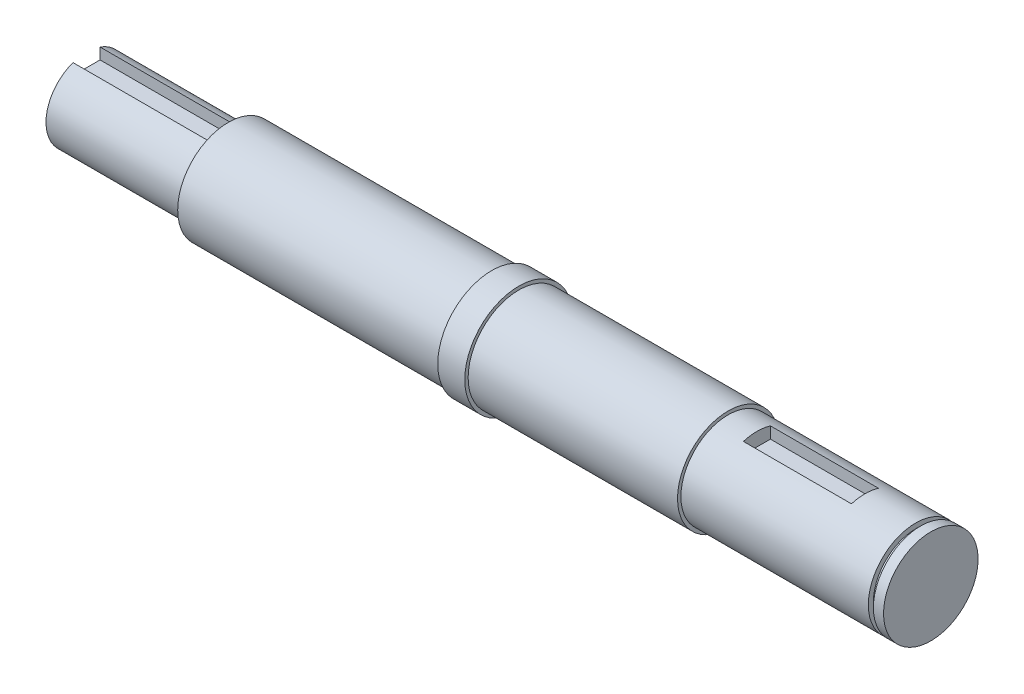
ISO-10303-21;
HEADER;
FILE_DESCRIPTION(('STEP AP214'),'2;1');
FILE_NAME('part.step','',(''),(''),'','','');
FILE_SCHEMA(('AUTOMOTIVE_DESIGN { 1 0 10303 214 1 1 1 1 }'));
ENDSEC;
DATA;
#1=APPLICATION_CONTEXT('core data for automotive mechanical design processes');
#2=APPLICATION_PROTOCOL_DEFINITION('international standard','automotive_design',2000,#1);
#3=PRODUCT_CONTEXT('',#1,'mechanical');
#4=PRODUCT('Part','Part','',(#3));
#5=PRODUCT_RELATED_PRODUCT_CATEGORY('part','',(#4));
#6=PRODUCT_DEFINITION_FORMATION('','',#4);
#7=PRODUCT_DEFINITION_CONTEXT('part definition',#1,'design');
#8=PRODUCT_DEFINITION('design','',#6,#7);
#9=PRODUCT_DEFINITION_SHAPE('','',#8);
#10=(LENGTH_UNIT() NAMED_UNIT(*) SI_UNIT(.MILLI.,.METRE.));
#11=(NAMED_UNIT(*) PLANE_ANGLE_UNIT() SI_UNIT($,.RADIAN.));
#12=(NAMED_UNIT(*) SI_UNIT($,.STERADIAN.) SOLID_ANGLE_UNIT());
#13=UNCERTAINTY_MEASURE_WITH_UNIT(LENGTH_MEASURE(1.E-05),#10,'distance_accuracy_value','');
#14=(GEOMETRIC_REPRESENTATION_CONTEXT(3) GLOBAL_UNCERTAINTY_ASSIGNED_CONTEXT((#13)) GLOBAL_UNIT_ASSIGNED_CONTEXT((#10,
#11,#12)) REPRESENTATION_CONTEXT('',''));
#15=CARTESIAN_POINT('',(0.,0.,0.));
#16=DIRECTION('',(0.,0.,1.));
#17=DIRECTION('',(1.,0.,0.));
#18=AXIS2_PLACEMENT_3D('',#15,#16,#17);
#19=CARTESIAN_POINT('',(0.,0.,0.));
#20=DIRECTION('',(1.,0.,0.));
#21=DIRECTION('',(0.,0.,-1.));
#22=AXIS2_PLACEMENT_3D('',#19,#20,#21);
#23=PLANE('',#22);
#24=DIRECTION('',(0.,0.,1.));
#25=VECTOR('',#24,1.);
#26=CARTESIAN_POINT('',(0.,8.,-4.));
#27=LINE('',#26,#25);
#28=CARTESIAN_POINT('',(0.,8.,-4.));
#29=VERTEX_POINT('',#28);
#30=CARTESIAN_POINT('',(0.,8.,4.));
#31=VERTEX_POINT('',#30);
#32=EDGE_CURVE('E128',#29,#31,#27,.T.);
#33=ORIENTED_EDGE('',*,*,#32,.F.);
#34=DIRECTION('',(0.,1.,0.));
#35=VECTOR('',#34,1.);
#36=CARTESIAN_POINT('',(0.,8.,-4.));
#37=LINE('',#36,#35);
#38=CARTESIAN_POINT('',(0.,11.3137084989848,-4.));
#39=VERTEX_POINT('',#38);
#40=EDGE_CURVE('E148',#29,#39,#37,.T.);
#41=ORIENTED_EDGE('',*,*,#40,.T.);
#42=CARTESIAN_POINT('',(0.,0.,0.));
#43=DIRECTION('',(-1.,0.,0.));
#44=DIRECTION('',(0.,0.,1.));
#45=AXIS2_PLACEMENT_3D('',#42,#43,#44);
#46=CIRCLE('',#45,12.);
#47=CARTESIAN_POINT('',(0.,11.3137084989848,4.));
#48=VERTEX_POINT('',#47);
#49=EDGE_CURVE('E200',#39,#48,#46,.T.);
#50=ORIENTED_EDGE('',*,*,#49,.T.);
#51=DIRECTION('',(0.,1.,0.));
#52=VECTOR('',#51,1.);
#53=CARTESIAN_POINT('',(0.,8.,4.));
#54=LINE('',#53,#52);
#55=EDGE_CURVE('E64',#31,#48,#54,.T.);
#56=ORIENTED_EDGE('',*,*,#55,.F.);
#57=EDGE_LOOP('',(#33,#41,#50,#56));
#58=FACE_BOUND('',#57,.T.);
#59=ADVANCED_FACE('F39',(#58),#23,.F.);
#60=CARTESIAN_POINT('',(0.,0.,0.));
#61=DIRECTION('',(-1.,0.,0.));
#62=DIRECTION('',(0.,0.,1.));
#63=AXIS2_PLACEMENT_3D('',#60,#61,#62);
#64=CYLINDRICAL_SURFACE('',#63,12.);
#65=ORIENTED_EDGE('',*,*,#49,.F.);
#66=DIRECTION('',(-1.,0.,0.));
#67=VECTOR('',#66,1.);
#68=CARTESIAN_POINT('',(0.,11.3137084989848,-4.));
#69=LINE('',#68,#67);
#70=CARTESIAN_POINT('',(42.,11.3137084989848,-4.));
#71=VERTEX_POINT('',#70);
#72=EDGE_CURVE('E160',#39,#71,#69,.F.);
#73=ORIENTED_EDGE('',*,*,#72,.T.);
#74=CARTESIAN_POINT('',(42.,0.,0.));
#75=DIRECTION('',(-1.,0.,0.));
#76=DIRECTION('',(0.,0.,1.));
#77=AXIS2_PLACEMENT_3D('',#74,#75,#76);
#78=CIRCLE('',#77,12.);
#79=CARTESIAN_POINT('',(42.,11.3137084989848,4.));
#80=VERTEX_POINT('',#79);
#81=EDGE_CURVE('E198',#71,#80,#78,.T.);
#82=ORIENTED_EDGE('',*,*,#81,.T.);
#83=DIRECTION('',(-1.,0.,0.));
#84=VECTOR('',#83,1.);
#85=CARTESIAN_POINT('',(0.,11.3137084989848,4.));
#86=LINE('',#85,#84);
#87=EDGE_CURVE('E149',#80,#48,#86,.T.);
#88=ORIENTED_EDGE('',*,*,#87,.T.);
#89=EDGE_LOOP('',(#65,#73,#82,#88));
#90=FACE_BOUND('',#89,.T.);
#91=ADVANCED_FACE('F224',(#90),#64,.T.);
#92=CARTESIAN_POINT('',(42.,12.,0.));
#93=DIRECTION('',(1.,0.,0.));
#94=DIRECTION('',(0.,0.,-1.));
#95=AXIS2_PLACEMENT_3D('',#92,#93,#94);
#96=PLANE('',#95);
#97=ORIENTED_EDGE('',*,*,#81,.F.);
#98=DIRECTION('',(0.,1.,0.));
#99=VECTOR('',#98,1.);
#100=CARTESIAN_POINT('',(42.,8.,-4.));
#101=LINE('',#100,#99);
#102=CARTESIAN_POINT('',(42.,8.,-4.));
#103=VERTEX_POINT('',#102);
#104=EDGE_CURVE('E147',#103,#71,#101,.T.);
#105=ORIENTED_EDGE('',*,*,#104,.F.);
#106=DIRECTION('',(0.,0.,-1.));
#107=VECTOR('',#106,1.);
#108=CARTESIAN_POINT('',(42.,8.,-4.));
#109=LINE('',#108,#107);
#110=CARTESIAN_POINT('',(42.,8.,4.));
#111=VERTEX_POINT('',#110);
#112=EDGE_CURVE('E139',#111,#103,#109,.T.);
#113=ORIENTED_EDGE('',*,*,#112,.F.);
#114=DIRECTION('',(0.,1.,0.));
#115=VECTOR('',#114,1.);
#116=CARTESIAN_POINT('',(42.,8.,4.));
#117=LINE('',#116,#115);
#118=EDGE_CURVE('E155',#111,#80,#117,.T.);
#119=ORIENTED_EDGE('',*,*,#118,.T.);
#120=EDGE_LOOP('',(#97,#105,#113,#119));
#121=FACE_BOUND('',#120,.T.);
#122=CARTESIAN_POINT('',(42.,0.,0.));
#123=DIRECTION('',(-1.,0.,0.));
#124=DIRECTION('',(0.,0.,1.));
#125=AXIS2_PLACEMENT_3D('',#122,#123,#124);
#126=CIRCLE('',#125,15.);
#127=CARTESIAN_POINT('',(42.,0.,15.));
#128=VERTEX_POINT('',#127);
#129=EDGE_CURVE('E193',#128,#128,#126,.T.);
#130=ORIENTED_EDGE('',*,*,#129,.T.);
#131=EDGE_LOOP('',(#130));
#132=FACE_BOUND('',#131,.T.);
#133=ADVANCED_FACE('F228',(#121,#132),#96,.F.);
#134=CARTESIAN_POINT('',(0.,0.,0.));
#135=DIRECTION('',(-1.,0.,0.));
#136=DIRECTION('',(0.,0.,1.));
#137=AXIS2_PLACEMENT_3D('',#134,#135,#136);
#138=CYLINDRICAL_SURFACE('',#137,15.);
#139=ORIENTED_EDGE('',*,*,#129,.F.);
#140=EDGE_LOOP('',(#139));
#141=FACE_BOUND('',#140,.T.);
#142=CARTESIAN_POINT('',(120.,0.,0.));
#143=DIRECTION('',(-1.,0.,0.));
#144=DIRECTION('',(0.,0.,1.));
#145=AXIS2_PLACEMENT_3D('',#142,#143,#144);
#146=CIRCLE('',#145,15.);
#147=CARTESIAN_POINT('',(120.,0.,15.));
#148=VERTEX_POINT('',#147);
#149=EDGE_CURVE('E187',#148,#148,#146,.T.);
#150=ORIENTED_EDGE('',*,*,#149,.T.);
#151=EDGE_LOOP('',(#150));
#152=FACE_BOUND('',#151,.T.);
#153=ADVANCED_FACE('F292',(#141,#152),#138,.T.);
#154=CARTESIAN_POINT('',(120.,15.,0.));
#155=DIRECTION('',(1.,0.,0.));
#156=DIRECTION('',(0.,0.,-1.));
#157=AXIS2_PLACEMENT_3D('',#154,#155,#156);
#158=PLANE('',#157);
#159=ORIENTED_EDGE('',*,*,#149,.F.);
#160=EDGE_LOOP('',(#159));
#161=FACE_BOUND('',#160,.T.);
#162=CARTESIAN_POINT('',(120.,0.,0.));
#163=DIRECTION('',(-1.,0.,0.));
#164=DIRECTION('',(0.,0.,1.));
#165=AXIS2_PLACEMENT_3D('',#162,#163,#164);
#166=CIRCLE('',#165,16.);
#167=CARTESIAN_POINT('',(120.,0.,16.));
#168=VERTEX_POINT('',#167);
#169=EDGE_CURVE('E186',#168,#168,#166,.T.);
#170=ORIENTED_EDGE('',*,*,#169,.T.);
#171=EDGE_LOOP('',(#170));
#172=FACE_BOUND('',#171,.T.);
#173=ADVANCED_FACE('F290',(#161,#172),#158,.F.);
#174=CARTESIAN_POINT('',(0.,0.,0.));
#175=DIRECTION('',(-1.,0.,0.));
#176=DIRECTION('',(0.,0.,1.));
#177=AXIS2_PLACEMENT_3D('',#174,#175,#176);
#178=CYLINDRICAL_SURFACE('',#177,16.);
#179=ORIENTED_EDGE('',*,*,#169,.F.);
#180=EDGE_LOOP('',(#179));
#181=FACE_BOUND('',#180,.T.);
#182=CARTESIAN_POINT('',(128.,0.,0.));
#183=DIRECTION('',(-1.,0.,0.));
#184=DIRECTION('',(0.,0.,1.));
#185=AXIS2_PLACEMENT_3D('',#182,#183,#184);
#186=CIRCLE('',#185,16.);
#187=CARTESIAN_POINT('',(128.,0.,16.));
#188=VERTEX_POINT('',#187);
#189=EDGE_CURVE('E184',#188,#188,#186,.T.);
#190=ORIENTED_EDGE('',*,*,#189,.T.);
#191=EDGE_LOOP('',(#190));
#192=FACE_BOUND('',#191,.T.);
#193=ADVANCED_FACE('F285',(#181,#192),#178,.T.);
#194=CARTESIAN_POINT('',(128.,16.,0.));
#195=DIRECTION('',(-1.,0.,0.));
#196=DIRECTION('',(0.,0.,1.));
#197=AXIS2_PLACEMENT_3D('',#194,#195,#196);
#198=PLANE('',#197);
#199=ORIENTED_EDGE('',*,*,#189,.F.);
#200=EDGE_LOOP('',(#199));
#201=FACE_BOUND('',#200,.T.);
#202=CARTESIAN_POINT('',(128.,0.,0.));
#203=DIRECTION('',(-1.,0.,0.));
#204=DIRECTION('',(0.,0.,1.));
#205=AXIS2_PLACEMENT_3D('',#202,#203,#204);
#206=CIRCLE('',#205,15.);
#207=CARTESIAN_POINT('',(128.,0.,15.));
#208=VERTEX_POINT('',#207);
#209=EDGE_CURVE('E182',#208,#208,#206,.T.);
#210=ORIENTED_EDGE('',*,*,#209,.T.);
#211=EDGE_LOOP('',(#210));
#212=FACE_BOUND('',#211,.T.);
#213=ADVANCED_FACE('F276',(#201,#212),#198,.F.);
#214=CARTESIAN_POINT('',(0.,0.,0.));
#215=DIRECTION('',(-1.,0.,0.));
#216=DIRECTION('',(0.,0.,1.));
#217=AXIS2_PLACEMENT_3D('',#214,#215,#216);
#218=CYLINDRICAL_SURFACE('',#217,15.);
#219=ORIENTED_EDGE('',*,*,#209,.F.);
#220=EDGE_LOOP('',(#219));
#221=FACE_BOUND('',#220,.T.);
#222=CARTESIAN_POINT('',(190.,0.,0.));
#223=DIRECTION('',(-1.,0.,0.));
#224=DIRECTION('',(0.,0.,1.));
#225=AXIS2_PLACEMENT_3D('',#222,#223,#224);
#226=CIRCLE('',#225,15.);
#227=CARTESIAN_POINT('',(190.,0.,15.));
#228=VERTEX_POINT('',#227);
#229=EDGE_CURVE('E178',#228,#228,#226,.T.);
#230=ORIENTED_EDGE('',*,*,#229,.T.);
#231=EDGE_LOOP('',(#230));
#232=FACE_BOUND('',#231,.T.);
#233=ADVANCED_FACE('F274',(#221,#232),#218,.T.);
#234=CARTESIAN_POINT('',(190.,15.,0.));
#235=DIRECTION('',(-1.,0.,0.));
#236=DIRECTION('',(0.,0.,1.));
#237=AXIS2_PLACEMENT_3D('',#234,#235,#236);
#238=PLANE('',#237);
#239=ORIENTED_EDGE('',*,*,#229,.F.);
#240=EDGE_LOOP('',(#239));
#241=FACE_BOUND('',#240,.T.);
#242=CARTESIAN_POINT('',(190.,0.,0.));
#243=DIRECTION('',(-1.,0.,0.));
#244=DIRECTION('',(0.,0.,1.));
#245=AXIS2_PLACEMENT_3D('',#242,#243,#244);
#246=CIRCLE('',#245,14.);
#247=CARTESIAN_POINT('',(190.,0.,14.));
#248=VERTEX_POINT('',#247);
#249=EDGE_CURVE('E172',#248,#248,#246,.T.);
#250=ORIENTED_EDGE('',*,*,#249,.T.);
#251=EDGE_LOOP('',(#250));
#252=FACE_BOUND('',#251,.T.);
#253=ADVANCED_FACE('F275',(#241,#252),#238,.F.);
#254=CARTESIAN_POINT('',(0.,0.,0.));
#255=DIRECTION('',(-1.,0.,0.));
#256=DIRECTION('',(0.,0.,1.));
#257=AXIS2_PLACEMENT_3D('',#254,#255,#256);
#258=CYLINDRICAL_SURFACE('',#257,14.);
#259=DIRECTION('',(-1.,0.,0.));
#260=VECTOR('',#259,1.);
#261=CARTESIAN_POINT('',(0.,13.4164078649988,-3.99999999999986));
#262=LINE('',#261,#260);
#263=CARTESIAN_POINT('',(198.5,13.4164078649988,-3.99999999999998));
#264=VERTEX_POINT('',#263);
#265=CARTESIAN_POINT('',(230.5,13.4164078649987,-3.99999999999999));
#266=VERTEX_POINT('',#265);
#267=EDGE_CURVE('E11',#264,#266,#262,.F.);
#268=ORIENTED_EDGE('',*,*,#267,.T.);
#269=CARTESIAN_POINT('',(230.5,0.,0.));
#270=DIRECTION('',(1.,0.,0.));
#271=DIRECTION('',(0.,0.,-1.));
#272=AXIS2_PLACEMENT_3D('',#269,#270,#271);
#273=CIRCLE('',#272,14.);
#274=CARTESIAN_POINT('',(230.5,13.4164078649987,4.00000000000001));
#275=VERTEX_POINT('',#274);
#276=EDGE_CURVE('E205',#266,#275,#273,.T.);
#277=ORIENTED_EDGE('',*,*,#276,.T.);
#278=DIRECTION('',(-1.,0.,0.));
#279=VECTOR('',#278,1.);
#280=CARTESIAN_POINT('',(0.,13.4164078649987,4.00000000000001));
#281=LINE('',#280,#279);
#282=CARTESIAN_POINT('',(198.5,13.4164078649987,4.00000000000001));
#283=VERTEX_POINT('',#282);
#284=EDGE_CURVE('E46',#275,#283,#281,.T.);
#285=ORIENTED_EDGE('',*,*,#284,.T.);
#286=CARTESIAN_POINT('',(198.5,0.,0.));
#287=DIRECTION('',(-1.,0.,0.));
#288=DIRECTION('',(0.,0.,1.));
#289=AXIS2_PLACEMENT_3D('',#286,#287,#288);
#290=CIRCLE('',#289,14.);
#291=EDGE_CURVE('E52',#283,#264,#290,.T.);
#292=ORIENTED_EDGE('',*,*,#291,.T.);
#293=EDGE_LOOP('',(#268,#277,#285,#292));
#294=FACE_BOUND('',#293,.T.);
#295=ORIENTED_EDGE('',*,*,#249,.F.);
#296=EDGE_LOOP('',(#295));
#297=FACE_BOUND('',#296,.T.);
#298=CARTESIAN_POINT('',(245.5,0.,0.));
#299=DIRECTION('',(-1.,0.,0.));
#300=DIRECTION('',(0.,0.,1.));
#301=AXIS2_PLACEMENT_3D('',#298,#299,#300);
#302=CIRCLE('',#301,14.);
#303=CARTESIAN_POINT('',(245.5,0.,14.));
#304=VERTEX_POINT('',#303);
#305=EDGE_CURVE('E171',#304,#304,#302,.T.);
#306=ORIENTED_EDGE('',*,*,#305,.T.);
#307=EDGE_LOOP('',(#306));
#308=FACE_BOUND('',#307,.T.);
#309=ADVANCED_FACE('F206',(#294,#297,#308),#258,.T.);
#310=CARTESIAN_POINT('',(245.5,14.,0.));
#311=DIRECTION('',(-1.,0.,0.));
#312=DIRECTION('',(0.,0.,1.));
#313=AXIS2_PLACEMENT_3D('',#310,#311,#312);
#314=PLANE('',#313);
#315=ORIENTED_EDGE('',*,*,#305,.F.);
#316=EDGE_LOOP('',(#315));
#317=FACE_BOUND('',#316,.T.);
#318=CARTESIAN_POINT('',(245.5,0.,0.));
#319=DIRECTION('',(-1.,0.,0.));
#320=DIRECTION('',(0.,0.,1.));
#321=AXIS2_PLACEMENT_3D('',#318,#319,#320);
#322=CIRCLE('',#321,12.5);
#323=CARTESIAN_POINT('',(245.5,0.,12.5));
#324=VERTEX_POINT('',#323);
#325=EDGE_CURVE('E166',#324,#324,#322,.T.);
#326=ORIENTED_EDGE('',*,*,#325,.T.);
#327=EDGE_LOOP('',(#326));
#328=FACE_BOUND('',#327,.T.);
#329=ADVANCED_FACE('F264',(#317,#328),#314,.F.);
#330=CARTESIAN_POINT('',(0.,0.,0.));
#331=DIRECTION('',(-1.,0.,0.));
#332=DIRECTION('',(0.,0.,1.));
#333=AXIS2_PLACEMENT_3D('',#330,#331,#332);
#334=CYLINDRICAL_SURFACE('',#333,12.5);
#335=ORIENTED_EDGE('',*,*,#325,.F.);
#336=EDGE_LOOP('',(#335));
#337=FACE_BOUND('',#336,.T.);
#338=CARTESIAN_POINT('',(247.,0.,0.));
#339=DIRECTION('',(-1.,0.,0.));
#340=DIRECTION('',(0.,0.,1.));
#341=AXIS2_PLACEMENT_3D('',#338,#339,#340);
#342=CIRCLE('',#341,12.5);
#343=CARTESIAN_POINT('',(247.,0.,12.5));
#344=VERTEX_POINT('',#343);
#345=EDGE_CURVE('E167',#344,#344,#342,.T.);
#346=ORIENTED_EDGE('',*,*,#345,.T.);
#347=EDGE_LOOP('',(#346));
#348=FACE_BOUND('',#347,.T.);
#349=ADVANCED_FACE('F261',(#337,#348),#334,.T.);
#350=CARTESIAN_POINT('',(247.,12.5,0.));
#351=DIRECTION('',(1.,0.,0.));
#352=DIRECTION('',(0.,0.,-1.));
#353=AXIS2_PLACEMENT_3D('',#350,#351,#352);
#354=PLANE('',#353);
#355=ORIENTED_EDGE('',*,*,#345,.F.);
#356=EDGE_LOOP('',(#355));
#357=FACE_BOUND('',#356,.T.);
#358=CARTESIAN_POINT('',(247.,0.,0.));
#359=DIRECTION('',(-1.,0.,0.));
#360=DIRECTION('',(0.,0.,1.));
#361=AXIS2_PLACEMENT_3D('',#358,#359,#360);
#362=CIRCLE('',#361,14.);
#363=CARTESIAN_POINT('',(247.,0.,14.));
#364=VERTEX_POINT('',#363);
#365=EDGE_CURVE('E162',#364,#364,#362,.T.);
#366=ORIENTED_EDGE('',*,*,#365,.T.);
#367=EDGE_LOOP('',(#366));
#368=FACE_BOUND('',#367,.T.);
#369=ADVANCED_FACE('F260',(#357,#368),#354,.F.);
#370=CARTESIAN_POINT('',(0.,0.,0.));
#371=DIRECTION('',(-1.,0.,0.));
#372=DIRECTION('',(0.,0.,1.));
#373=AXIS2_PLACEMENT_3D('',#370,#371,#372);
#374=CYLINDRICAL_SURFACE('',#373,14.);
#375=ORIENTED_EDGE('',*,*,#365,.F.);
#376=EDGE_LOOP('',(#375));
#377=FACE_BOUND('',#376,.T.);
#378=CARTESIAN_POINT('',(250.,0.,0.));
#379=DIRECTION('',(-1.,0.,0.));
#380=DIRECTION('',(0.,0.,1.));
#381=AXIS2_PLACEMENT_3D('',#378,#379,#380);
#382=CIRCLE('',#381,14.);
#383=CARTESIAN_POINT('',(250.,0.,14.));
#384=VERTEX_POINT('',#383);
#385=EDGE_CURVE('E159',#384,#384,#382,.T.);
#386=ORIENTED_EDGE('',*,*,#385,.T.);
#387=EDGE_LOOP('',(#386));
#388=FACE_BOUND('',#387,.T.);
#389=ADVANCED_FACE('F251',(#377,#388),#374,.T.);
#390=CARTESIAN_POINT('',(250.,14.,0.));
#391=DIRECTION('',(-1.,0.,0.));
#392=DIRECTION('',(0.,0.,1.));
#393=AXIS2_PLACEMENT_3D('',#390,#391,#392);
#394=PLANE('',#393);
#395=ORIENTED_EDGE('',*,*,#385,.F.);
#396=EDGE_LOOP('',(#395));
#397=FACE_BOUND('',#396,.T.);
#398=ADVANCED_FACE('F247',(#397),#394,.F.);
#399=CARTESIAN_POINT('',(0.,8.,-4.));
#400=DIRECTION('',(0.,0.,-1.));
#401=DIRECTION('',(-1.,0.,0.));
#402=AXIS2_PLACEMENT_3D('',#399,#400,#401);
#403=PLANE('',#402);
#404=ORIENTED_EDGE('',*,*,#40,.F.);
#405=DIRECTION('',(-1.,0.,0.));
#406=VECTOR('',#405,1.);
#407=CARTESIAN_POINT('',(0.,8.,-4.));
#408=LINE('',#407,#406);
#409=EDGE_CURVE('E141',#103,#29,#408,.T.);
#410=ORIENTED_EDGE('',*,*,#409,.F.);
#411=ORIENTED_EDGE('',*,*,#104,.T.);
#412=ORIENTED_EDGE('',*,*,#72,.F.);
#413=EDGE_LOOP('',(#404,#410,#411,#412));
#414=FACE_BOUND('',#413,.T.);
#415=ADVANCED_FACE('F240',(#414),#403,.F.);
#416=CARTESIAN_POINT('',(0.,8.,4.));
#417=DIRECTION('',(0.,0.,1.));
#418=DIRECTION('',(1.,0.,0.));
#419=AXIS2_PLACEMENT_3D('',#416,#417,#418);
#420=PLANE('',#419);
#421=ORIENTED_EDGE('',*,*,#118,.F.);
#422=DIRECTION('',(1.,0.,0.));
#423=VECTOR('',#422,1.);
#424=CARTESIAN_POINT('',(0.,8.,4.));
#425=LINE('',#424,#423);
#426=EDGE_CURVE('E140',#31,#111,#425,.T.);
#427=ORIENTED_EDGE('',*,*,#426,.F.);
#428=ORIENTED_EDGE('',*,*,#55,.T.);
#429=ORIENTED_EDGE('',*,*,#87,.F.);
#430=EDGE_LOOP('',(#421,#427,#428,#429));
#431=FACE_BOUND('',#430,.T.);
#432=ADVANCED_FACE('F244',(#431),#420,.F.);
#433=CARTESIAN_POINT('',(0.,8.,0.));
#434=DIRECTION('',(0.,1.,0.));
#435=DIRECTION('',(0.,0.,1.));
#436=AXIS2_PLACEMENT_3D('',#433,#434,#435);
#437=PLANE('',#436);
#438=ORIENTED_EDGE('',*,*,#32,.T.);
#439=ORIENTED_EDGE('',*,*,#426,.T.);
#440=ORIENTED_EDGE('',*,*,#112,.T.);
#441=ORIENTED_EDGE('',*,*,#409,.T.);
#442=EDGE_LOOP('',(#438,#439,#440,#441));
#443=FACE_BOUND('',#442,.T.);
#444=ADVANCED_FACE('F218',(#443),#437,.T.);
#445=CARTESIAN_POINT('',(198.5,10.,-3.99999999999998));
#446=DIRECTION('',(-1.,0.,0.));
#447=DIRECTION('',(0.,0.,1.));
#448=AXIS2_PLACEMENT_3D('',#445,#446,#447);
#449=PLANE('',#448);
#450=DIRECTION('',(0.,1.,0.));
#451=VECTOR('',#450,1.);
#452=CARTESIAN_POINT('',(198.5,10.,4.00000000000001));
#453=LINE('',#452,#451);
#454=CARTESIAN_POINT('',(198.5,10.,4.00000000000001));
#455=VERTEX_POINT('',#454);
#456=EDGE_CURVE('E105',#455,#283,#453,.T.);
#457=ORIENTED_EDGE('',*,*,#456,.F.);
#458=DIRECTION('',(0.,0.,1.));
#459=VECTOR('',#458,1.);
#460=CARTESIAN_POINT('',(198.5,10.,-3.99999999999998));
#461=LINE('',#460,#459);
#462=CARTESIAN_POINT('',(198.5,10.,-3.99999999999998));
#463=VERTEX_POINT('',#462);
#464=EDGE_CURVE('E106',#463,#455,#461,.T.);
#465=ORIENTED_EDGE('',*,*,#464,.F.);
#466=DIRECTION('',(0.,1.,0.));
#467=VECTOR('',#466,1.);
#468=CARTESIAN_POINT('',(198.5,10.,-3.99999999999998));
#469=LINE('',#468,#467);
#470=EDGE_CURVE('E126',#463,#264,#469,.T.);
#471=ORIENTED_EDGE('',*,*,#470,.T.);
#472=ORIENTED_EDGE('',*,*,#291,.F.);
#473=EDGE_LOOP('',(#457,#465,#471,#472));
#474=FACE_BOUND('',#473,.T.);
#475=ADVANCED_FACE('F102',(#474),#449,.F.);
#476=CARTESIAN_POINT('',(198.5,10.,-3.99999999999998));
#477=DIRECTION('',(0.,0.,-1.));
#478=DIRECTION('',(-1.,0.,0.));
#479=AXIS2_PLACEMENT_3D('',#476,#477,#478);
#480=PLANE('',#479);
#481=ORIENTED_EDGE('',*,*,#470,.F.);
#482=DIRECTION('',(-1.,0.,0.));
#483=VECTOR('',#482,1.);
#484=CARTESIAN_POINT('',(198.5,10.,-3.99999999999998));
#485=LINE('',#484,#483);
#486=CARTESIAN_POINT('',(230.5,10.,-3.99999999999999));
#487=VERTEX_POINT('',#486);
#488=EDGE_CURVE('E112',#487,#463,#485,.T.);
#489=ORIENTED_EDGE('',*,*,#488,.F.);
#490=DIRECTION('',(0.,1.,0.));
#491=VECTOR('',#490,1.);
#492=CARTESIAN_POINT('',(230.5,10.,-3.99999999999999));
#493=LINE('',#492,#491);
#494=EDGE_CURVE('E134',#487,#266,#493,.T.);
#495=ORIENTED_EDGE('',*,*,#494,.T.);
#496=ORIENTED_EDGE('',*,*,#267,.F.);
#497=EDGE_LOOP('',(#481,#489,#495,#496));
#498=FACE_BOUND('',#497,.T.);
#499=ADVANCED_FACE('F211',(#498),#480,.F.);
#500=CARTESIAN_POINT('',(230.5,10.,-3.99999999999999));
#501=DIRECTION('',(1.,0.,0.));
#502=DIRECTION('',(0.,0.,-1.));
#503=AXIS2_PLACEMENT_3D('',#500,#501,#502);
#504=PLANE('',#503);
#505=ORIENTED_EDGE('',*,*,#494,.F.);
#506=DIRECTION('',(0.,0.,-1.));
#507=VECTOR('',#506,1.);
#508=CARTESIAN_POINT('',(230.5,10.,-3.99999999999999));
#509=LINE('',#508,#507);
#510=CARTESIAN_POINT('',(230.5,10.,4.00000000000001));
#511=VERTEX_POINT('',#510);
#512=EDGE_CURVE('E117',#511,#487,#509,.T.);
#513=ORIENTED_EDGE('',*,*,#512,.F.);
#514=DIRECTION('',(0.,1.,0.));
#515=VECTOR('',#514,1.);
#516=CARTESIAN_POINT('',(230.5,10.,4.00000000000001));
#517=LINE('',#516,#515);
#518=EDGE_CURVE('E109',#511,#275,#517,.T.);
#519=ORIENTED_EDGE('',*,*,#518,.T.);
#520=ORIENTED_EDGE('',*,*,#276,.F.);
#521=EDGE_LOOP('',(#505,#513,#519,#520));
#522=FACE_BOUND('',#521,.T.);
#523=ADVANCED_FACE('F207',(#522),#504,.F.);
#524=CARTESIAN_POINT('',(198.5,10.,4.00000000000001));
#525=DIRECTION('',(0.,0.,1.));
#526=DIRECTION('',(1.,0.,0.));
#527=AXIS2_PLACEMENT_3D('',#524,#525,#526);
#528=PLANE('',#527);
#529=ORIENTED_EDGE('',*,*,#518,.F.);
#530=DIRECTION('',(1.,0.,0.));
#531=VECTOR('',#530,1.);
#532=CARTESIAN_POINT('',(198.5,10.,4.00000000000001));
#533=LINE('',#532,#531);
#534=EDGE_CURVE('E111',#455,#511,#533,.T.);
#535=ORIENTED_EDGE('',*,*,#534,.F.);
#536=ORIENTED_EDGE('',*,*,#456,.T.);
#537=ORIENTED_EDGE('',*,*,#284,.F.);
#538=EDGE_LOOP('',(#529,#535,#536,#537));
#539=FACE_BOUND('',#538,.T.);
#540=ADVANCED_FACE('F113',(#539),#528,.F.);
#541=CARTESIAN_POINT('',(0.,10.,0.));
#542=DIRECTION('',(0.,1.,0.));
#543=DIRECTION('',(0.,0.,1.));
#544=AXIS2_PLACEMENT_3D('',#541,#542,#543);
#545=PLANE('',#544);
#546=ORIENTED_EDGE('',*,*,#464,.T.);
#547=ORIENTED_EDGE('',*,*,#534,.T.);
#548=ORIENTED_EDGE('',*,*,#512,.T.);
#549=ORIENTED_EDGE('',*,*,#488,.T.);
#550=EDGE_LOOP('',(#546,#547,#548,#549));
#551=FACE_BOUND('',#550,.T.);
#552=ADVANCED_FACE('F125',(#551),#545,.T.);
#553=CLOSED_SHELL('',(#59,#91,#133,#153,#173,#193,#213,#233,#253,#309,#329,#349,#369,#389,#398,
#415,#432,#444,#475,#499,#523,#540,#552));
#554=MANIFOLD_SOLID_BREP('B2',#553);
#555=ADVANCED_BREP_SHAPE_REPRESENTATION('',(#18,#554),#14);
#556=SHAPE_DEFINITION_REPRESENTATION(#9,#555);
ENDSEC;
END-ISO-10303-21;
